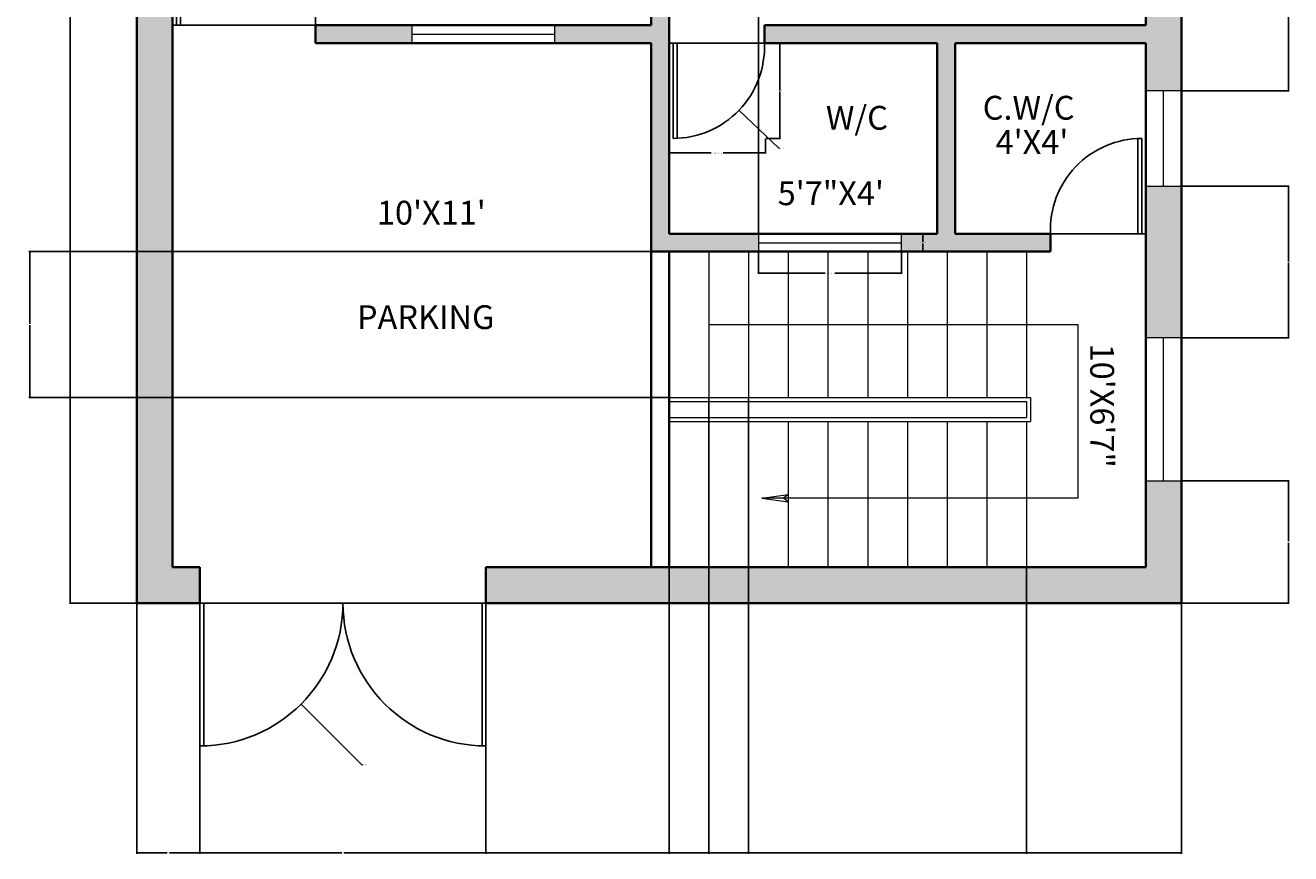
# Model space of a CAD drawing. Units: inches. Extents: x 2 to 321, y -521 to 41.
# Tile 1 of 2: x 2 to 321, y -521 to -312. Entities that reach past the tile are written whole.
import ezdxf

# ---------------------------------------------------------------- set-up
doc = ezdxf.new("R2010")
doc.units = ezdxf.units.IN
doc.header["$MEASUREMENT"] = 0
for name, color, linetype, lineweight in [('A-ANNO-DIMS', 2, 'Continuous', 18), ('A-ANNO-TEXT', 22, 'Continuous', 18), ('A-AREA-IDEN', 102, 'Continuous', 25), ('A-DOOR', 3, 'Continuous', 25), ('A-FLOR-STRS', 7, 'Continuous', 18), ('A-GLAZ', 4, 'Continuous', 18), ('A-WALL', 7, 'Continuous', 35), ('A-WALL-PATT', 5, 'Continuous', 13)]:
    doc.layers.add(name, color=color, linetype=linetype, lineweight=lineweight)
doc.styles.get("Standard").update_dxf_attribs({"font": 'arial.ttf'})
doc.dimstyles.get("Standard").update_dxf_attribs({"dimtxt": 0.18, "dimasz": 0.18, "dimexe": 0.18, "dimexo": 0.0625, "dimgap": 0.09, "dimtad": 0, "dimtih": 1, "dimtoh": 1, "dimdec": 0, "dimzin": 0, "dimdsep": 46, "dimlunit": 3, "dimtxsty": 'Standard', "dimcen": 0.09, "dimadec": 0, "dimazin": 0, "dimtfac": 1, "dimtdec": 0, "dimtofl": 0, "dimtmove": 0, "dimatfit": 3, "dimfxl": 1, "dimtolj": 1, "dimtzin": 0, "dimarcsym": 0})

# ---------------------------------------------------------------- blocks, each defined once
blk = doc.blocks.new('*D2')
at = {"layer": 'A-ANNO-DIMS', "color": 0, "lineweight": -2, "transparency": 16777216}
for p, q in [((30.1, 14.04), (13.23, 14.04)), ((13.41, 13.86), (13.41, -218.56)), ((13.41, -457.28), (13.41, -224.87)), ((30.1, -457.46), (13.23, -457.46))]:
    blk.add_line(p, q, dxfattribs=at)
at = {"layer": 'A-ANNO-DIMS', "color": 0, "transparency": 16777216}
for points in [[(13.38, 13.86), (13.44, 13.86), (13.41, 14.04)], [(13.38, -457.28), (13.44, -457.28), (13.41, -457.46)]]:
    blk.add_solid(points, dxfattribs=at)
at = {"layer": 'Defpoints', "color": 0, "transparency": 16777216}
for p in [(30.16, 14.04), (13.41, -457.46), (30.16, -457.46)]:
    blk.add_point(p, dxfattribs=at)
at = {"layer": 'A-ANNO-DIMS', "color": 0, "transparency": 16777216, "insert": (13.41, -221.71), "char_height": 6, "attachment_point": 5}
blk.add_mtext('\\A1;39\'-4"', dxfattribs=at)
blk = doc.blocks.new('WIN-36IN-9IN-WALL')
for p, q in [((0, 36), (0, 0)), ((9, 36), (0, 36)), ((4.5, 36), (4.5, 0)), ((9, 0), (9, 36)), ((0, 0), (9, 0))]:
    blk.add_line(p, q)
blk = doc.blocks.new('WIN-36IN-4_5IN-WALL')
for p, q in [((0, 4.5), (0, 0)), ((36, 4.5), (0, 4.5)), ((36, 0), (36, 4.5)), ((0, 2.25), (36, 2.25)), ((0, 0), (36, 0))]:
    blk.add_line(p, q)
blk = doc.blocks.new('WIN-24IN-9IN-WALL')
for p, q in [((0, 24), (0, 0)), ((9, 24), (0, 24)), ((4.5, 24), (4.5, 0)), ((9, 0), (9, 24)), ((0, 0), (9, 0))]:
    blk.add_line(p, q)
blk = doc.blocks.new('DOOR-SINGLE-36IN')
for p, q in [((1, 0), (1, 36)), ((2, 0), (2, 36)), ((36, 0), (0, 0))]:
    blk.add_line(p, q)
blk.add_arc((1, 0.99), 35.01, 358.3861, 90)
blk = doc.blocks.new('DOOR-SINGLE-24IN')
for p, q in [((24, 24), (0, 24)), ((1, 24), (1, 0)), ((2, 24), (2, 0))]:
    blk.add_line(p, q)
blk.add_arc((1, 23.02), 23.02, 270, 2.4378)
blk = doc.blocks.new('*D12')
at = {"layer": 'A-ANNO-DIMS', "color": 0, "lineweight": -2, "transparency": 16777216}
for p, q in [((186.66, -369.03), (186.66, -374.54)), ((222.66, -369.03), (222.66, -374.54)), ((186.84, -374.36), (203.43, -374.36)), ((222.48, -374.36), (205.88, -374.36))]:
    blk.add_line(p, q, dxfattribs=at)
at = {"layer": 'A-ANNO-DIMS', "color": 0, "transparency": 16777216}
for points in [[(186.84, -374.33), (186.84, -374.39), (186.66, -374.36)], [(222.48, -374.33), (222.48, -374.39), (222.66, -374.36)]]:
    blk.add_solid(points, dxfattribs=at)
at = {"layer": 'Defpoints', "color": 0, "transparency": 16777216}
for p in [(186.66, -368.96), (222.66, -368.96), (222.66, -374.36)]:
    blk.add_point(p, dxfattribs=at)
at = {"layer": 'A-ANNO-DIMS', "color": 0, "transparency": 16777216, "insert": (204.66, -374.36), "char_height": 0.18, "attachment_point": 5}
blk.add_mtext('\\A1;WINDOW 3\'-0" TYP.', dxfattribs=at)
blk = doc.blocks.new('*D13')
at = {"layer": 'A-ANNO-DIMS', "color": 0, "lineweight": -2, "transparency": 16777216}
for p, q in [((222.72, -364.46), (228.24, -364.46)), ((228.06, -364.64), (228.06, -366.53)), ((222.72, -368.96), (228.24, -368.96)), ((228.06, -368.78), (228.06, -366.9))]:
    blk.add_line(p, q, dxfattribs=at)
at = {"layer": 'A-ANNO-DIMS', "color": 0, "transparency": 16777216}
for points in [[(228.03, -364.64), (228.09, -364.64), (228.06, -364.46)], [(228.03, -368.78), (228.09, -368.78), (228.06, -368.96)]]:
    blk.add_solid(points, dxfattribs=at)
at = {"layer": 'Defpoints', "color": 0, "transparency": 16777216}
for p in [(222.66, -364.46), (228.06, -364.46), (222.66, -368.96)]:
    blk.add_point(p, dxfattribs=at)
at = {"layer": 'A-ANNO-DIMS', "color": 0, "transparency": 16777216, "insert": (228.06, -366.71), "char_height": 0.18, "attachment_point": 5}
blk.add_mtext('\\A1;0\'-4 1/2" TYP.', dxfattribs=at)
blk = doc.blocks.new('*D16')
at = {"layer": 'A-ANNO-DIMS', "color": 0, "lineweight": -2, "transparency": 16777216}
for p, q in [((164.16, -340.53), (164.16, -344.28)), ((188.43, -340.53), (188.43, -344.28)), ((164.34, -344.1), (174.79, -344.1)), ((188.25, -344.1), (177.8, -344.1))]:
    blk.add_line(p, q, dxfattribs=at)
at = {"layer": 'A-ANNO-DIMS', "color": 0, "transparency": 16777216}
for points in [[(164.34, -344.07), (164.34, -344.13), (164.16, -344.1)], [(188.25, -344.07), (188.25, -344.13), (188.43, -344.1)]]:
    blk.add_solid(points, dxfattribs=at)
at = {"layer": 'Defpoints', "color": 0, "transparency": 16777216}
for p in [(164.16, -340.46), (188.43, -340.46), (188.43, -344.1)]:
    blk.add_point(p, dxfattribs=at)
at = {"layer": 'A-ANNO-DIMS', "color": 0, "transparency": 16777216, "insert": (176.29, -344.1), "char_height": 0.18, "attachment_point": 5}
blk.add_mtext('\\A1;WC DOOR 2\'-0 1/2" TYP.', dxfattribs=at)
blk = doc.blocks.new('*D17')
at = {"layer": 'A-ANNO-DIMS', "color": 0, "lineweight": -2, "transparency": 16777216}
for p, q in [((188.49, -316.46), (192.25, -316.46)), ((192.07, -316.64), (192.07, -328.28)), ((192.07, -340.28), (192.07, -328.65)), ((188.49, -340.46), (192.25, -340.46))]:
    blk.add_line(p, q, dxfattribs=at)
at = {"layer": 'A-ANNO-DIMS', "color": 0, "transparency": 16777216}
for points in [[(192.04, -316.64), (192.1, -316.64), (192.07, -316.46)], [(192.04, -340.28), (192.1, -340.28), (192.07, -340.46)]]:
    blk.add_solid(points, dxfattribs=at)
at = {"layer": 'Defpoints', "color": 0, "transparency": 16777216}
for p in [(188.43, -316.46), (192.07, -316.46), (188.43, -340.46)]:
    blk.add_point(p, dxfattribs=at)
at = {"layer": 'A-ANNO-DIMS', "color": 0, "transparency": 16777216, "insert": (192.07, -328.46), "char_height": 0.18, "attachment_point": 5}
blk.add_mtext('\\A1;2\'-0" TYP.', dxfattribs=at)
blk = doc.blocks.new('*D18')
at = {"layer": 'A-ANNO-DIMS', "color": 0, "lineweight": -2, "transparency": 16777216}
for p, q in [((30.16, -457.53), (30.16, -520.59)), ((46.07, -457.53), (46.07, -520.59)), ((30.34, -520.41), (37.8, -520.41)), ((45.89, -520.41), (38.44, -520.41))]:
    blk.add_line(p, q, dxfattribs=at)
at = {"layer": 'A-ANNO-DIMS', "color": 0, "transparency": 16777216}
for points in [[(30.34, -520.38), (30.34, -520.44), (30.16, -520.41)], [(45.89, -520.38), (45.89, -520.44), (46.07, -520.41)]]:
    blk.add_solid(points, dxfattribs=at)
at = {"layer": 'Defpoints', "color": 0, "transparency": 16777216}
for p in [(30.16, -457.46), (46.07, -457.46), (46.07, -520.41)]:
    blk.add_point(p, dxfattribs=at)
at = {"layer": 'A-ANNO-DIMS', "color": 0, "transparency": 16777216, "insert": (38.12, -520.41), "char_height": 0.18, "attachment_point": 5}
blk.add_mtext('\\A1;1\'-4"', dxfattribs=at)
blk = doc.blocks.new('*D19')
at = {"layer": 'A-ANNO-DIMS', "color": 0, "lineweight": -2, "transparency": 16777216}
for p, q in [((46.07, -457.53), (46.07, -520.59)), ((118.07, -457.53), (118.07, -520.59)), ((46.25, -520.41), (81.75, -520.41)), ((117.89, -520.41), (82.4, -520.41))]:
    blk.add_line(p, q, dxfattribs=at)
at = {"layer": 'A-ANNO-DIMS', "color": 0, "transparency": 16777216}
for points in [[(46.25, -520.38), (46.25, -520.44), (46.07, -520.41)], [(117.89, -520.38), (117.89, -520.44), (118.07, -520.41)]]:
    blk.add_solid(points, dxfattribs=at)
at = {"layer": 'Defpoints', "color": 0, "transparency": 16777216}
for p in [(46.07, -457.46), (118.07, -457.46), (118.07, -520.41)]:
    blk.add_point(p, dxfattribs=at)
at = {"layer": 'A-ANNO-DIMS', "color": 0, "transparency": 16777216, "insert": (82.07, -520.41), "char_height": 0.18, "attachment_point": 5}
blk.add_mtext('\\A1;6\'-0"', dxfattribs=at)
blk = doc.blocks.new('*D20')
at = {"layer": 'A-ANNO-DIMS', "color": 0, "lineweight": -2, "transparency": 16777216}
for p, q in [((118.07, -457.53), (118.07, -520.59)), ((293.16, -457.53), (293.16, -520.59)), ((118.25, -520.41), (205.23, -520.41)), ((292.98, -520.41), (206.01, -520.41))]:
    blk.add_line(p, q, dxfattribs=at)
at = {"layer": 'A-ANNO-DIMS', "color": 0, "transparency": 16777216}
for points in [[(118.25, -520.38), (118.25, -520.44), (118.07, -520.41)], [(292.98, -520.38), (292.98, -520.44), (293.16, -520.41)]]:
    blk.add_solid(points, dxfattribs=at)
at = {"layer": 'Defpoints', "color": 0, "transparency": 16777216}
for p in [(118.07, -457.46), (293.16, -457.46), (293.16, -520.41)]:
    blk.add_point(p, dxfattribs=at)
at = {"layer": 'A-ANNO-DIMS', "color": 0, "transparency": 16777216, "insert": (205.62, -520.41), "char_height": 0.18, "attachment_point": 5}
blk.add_mtext('\\A1;14\'-7"', dxfattribs=at)
blk = doc.blocks.new('*D26')
at = {"layer": 'A-ANNO-DIMS', "color": 0, "lineweight": -2, "transparency": 16777216}
for p, q in [((293.22, -269.96), (320.29, -269.96)), ((320.11, -270.14), (320.11, -299.03)), ((320.11, -328.28), (320.11, -299.4)), ((293.22, -328.46), (320.29, -328.46))]:
    blk.add_line(p, q, dxfattribs=at)
at = {"layer": 'A-ANNO-DIMS', "color": 0, "transparency": 16777216}
for points in [[(320.08, -270.14), (320.14, -270.14), (320.11, -269.96)], [(320.08, -328.28), (320.14, -328.28), (320.11, -328.46)]]:
    blk.add_solid(points, dxfattribs=at)
at = {"layer": 'Defpoints', "color": 0, "transparency": 16777216}
for p in [(293.16, -269.96), (293.16, -328.46), (320.11, -328.46)]:
    blk.add_point(p, dxfattribs=at)
at = {"layer": 'A-ANNO-DIMS', "color": 0, "transparency": 16777216, "insert": (320.11, -299.21), "char_height": 0.18, "attachment_point": 5}
blk.add_mtext('\\A1;4\'-10 1/2"', dxfattribs=at)
blk = doc.blocks.new('*D27')
at = {"layer": 'A-ANNO-DIMS', "color": 0, "lineweight": -2, "transparency": 16777216}
for p, q in [((293.22, -352.46), (320.29, -352.46)), ((320.11, -352.64), (320.11, -371.41)), ((320.11, -390.53), (320.11, -371.77)), ((293.22, -390.71), (320.29, -390.71))]:
    blk.add_line(p, q, dxfattribs=at)
at = {"layer": 'A-ANNO-DIMS', "color": 0, "transparency": 16777216}
for points in [[(320.08, -352.64), (320.14, -352.64), (320.11, -352.46)], [(320.08, -390.53), (320.14, -390.53), (320.11, -390.71)]]:
    blk.add_solid(points, dxfattribs=at)
at = {"layer": 'Defpoints', "color": 0, "transparency": 16777216}
for p in [(293.16, -352.46), (293.16, -390.71), (320.11, -390.71)]:
    blk.add_point(p, dxfattribs=at)
at = {"layer": 'A-ANNO-DIMS', "color": 0, "transparency": 16777216, "insert": (320.11, -371.59), "char_height": 0.18, "attachment_point": 5}
blk.add_mtext('\\A1;3\'-2 1/2"', dxfattribs=at)
blk = doc.blocks.new('*D28')
at = {"layer": 'A-ANNO-DIMS', "color": 0, "lineweight": -2, "transparency": 16777216}
for p, q in [((293.22, -426.71), (320.29, -426.71)), ((320.11, -426.89), (320.11, -441.91)), ((320.11, -457.28), (320.11, -442.27)), ((293.22, -457.46), (320.29, -457.46))]:
    blk.add_line(p, q, dxfattribs=at)
at = {"layer": 'A-ANNO-DIMS', "color": 0, "transparency": 16777216}
for points in [[(320.08, -426.89), (320.14, -426.89), (320.11, -426.71)], [(320.08, -457.28), (320.14, -457.28), (320.11, -457.46)]]:
    blk.add_solid(points, dxfattribs=at)
at = {"layer": 'Defpoints', "color": 0, "transparency": 16777216}
for p in [(293.16, -426.71), (293.16, -457.46), (320.11, -457.46)]:
    blk.add_point(p, dxfattribs=at)
at = {"layer": 'A-ANNO-DIMS', "color": 0, "transparency": 16777216, "insert": (320.11, -442.09), "char_height": 0.18, "attachment_point": 5}
blk.add_mtext('\\A1;2\'-7"', dxfattribs=at)
blk = doc.blocks.new('*D30')
at = {"layer": 'A-ANNO-DIMS', "color": 0, "lineweight": -2, "transparency": 16777216}
for p, q in [((164.16, -364.4), (164.16, 41.17)), ((164.34, 40.99), (174.81, 40.99)), ((186.48, 40.99), (176.01, 40.99)), ((186.66, -364.4), (186.66, 41.17))]:
    blk.add_line(p, q, dxfattribs=at)
at = {"layer": 'A-ANNO-DIMS', "color": 0, "transparency": 16777216}
for points in [[(164.34, 41.02), (164.34, 40.96), (164.16, 40.99)], [(186.48, 41.02), (186.48, 40.96), (186.66, 40.99)]]:
    blk.add_solid(points, dxfattribs=at)
at = {"layer": 'Defpoints', "color": 0, "transparency": 16777216}
for p in [(186.66, 40.99), (164.16, -364.46), (186.66, -364.46)]:
    blk.add_point(p, dxfattribs=at)
at = {"layer": 'A-ANNO-DIMS', "color": 0, "transparency": 16777216, "insert": (175.41, 40.99), "char_height": 0.18, "attachment_point": 5}
blk.add_mtext('\\A1;1\'-10 1/2"', dxfattribs=at)
blk = doc.blocks.new('*D31')
at = {"layer": 'A-ANNO-DIMS', "color": 0, "lineweight": -2, "transparency": 16777216}
for p, q in [((164.16, -448.53), (164.16, -520.59)), ((254.16, -448.53), (254.16, -520.59)), ((164.34, -520.41), (208.83, -520.41)), ((253.98, -520.41), (209.49, -520.41))]:
    blk.add_line(p, q, dxfattribs=at)
at = {"layer": 'A-ANNO-DIMS', "color": 0, "transparency": 16777216}
for points in [[(164.34, -520.38), (164.34, -520.44), (164.16, -520.41)], [(253.98, -520.38), (253.98, -520.44), (254.16, -520.41)]]:
    blk.add_solid(points, dxfattribs=at)
at = {"layer": 'Defpoints', "color": 0, "transparency": 16777216}
for p in [(164.16, -448.46), (254.16, -448.46), (254.16, -520.41)]:
    blk.add_point(p, dxfattribs=at)
at = {"layer": 'A-ANNO-DIMS', "color": 0, "transparency": 16777216, "insert": (209.16, -520.41), "char_height": 0.18, "attachment_point": 5}
blk.add_mtext('\\A1;7\'-6"', dxfattribs=at)
blk = doc.blocks.new('*D32')
at = {"layer": 'A-ANNO-DIMS', "color": 0, "lineweight": -2, "transparency": 16777216}
for p, q in [((174.16, -405.78), (174.16, -520.59)), ((184.16, -405.78), (184.16, -520.59)), ((174.34, -520.41), (178.76, -520.41)), ((183.98, -520.41), (179.56, -520.41))]:
    blk.add_line(p, q, dxfattribs=at)
at = {"layer": 'A-ANNO-DIMS', "color": 0, "transparency": 16777216}
for points in [[(174.34, -520.38), (174.34, -520.44), (174.16, -520.41)], [(183.98, -520.38), (183.98, -520.44), (184.16, -520.41)]]:
    blk.add_solid(points, dxfattribs=at)
at = {"layer": 'Defpoints', "color": 0, "transparency": 16777216}
for p in [(174.16, -405.71), (184.16, -405.71), (184.16, -520.41)]:
    blk.add_point(p, dxfattribs=at)
at = {"layer": 'A-ANNO-DIMS', "color": 0, "transparency": 16777216, "insert": (179.16, -520.41), "char_height": 0.18, "attachment_point": 5}
blk.add_mtext('\\A1;0\'-10"', dxfattribs=at)
blk = doc.blocks.new('*D33')
at = {"layer": 'A-ANNO-DIMS', "color": 0, "lineweight": -2, "transparency": 16777216}
for p, q in [((164.1, -368.96), (3.03, -368.96)), ((3.21, -369.14), (3.21, -387.16)), ((3.21, -405.53), (3.21, -387.52)), ((164.1, -405.71), (3.03, -405.71))]:
    blk.add_line(p, q, dxfattribs=at)
at = {"layer": 'A-ANNO-DIMS', "color": 0, "transparency": 16777216}
for points in [[(3.18, -369.14), (3.24, -369.14), (3.21, -368.96)], [(3.18, -405.53), (3.24, -405.53), (3.21, -405.71)]]:
    blk.add_solid(points, dxfattribs=at)
at = {"layer": 'Defpoints', "color": 0, "transparency": 16777216}
for p in [(3.21, -368.96), (164.16, -368.96), (164.16, -405.71)]:
    blk.add_point(p, dxfattribs=at)
at = {"layer": 'A-ANNO-DIMS', "color": 0, "transparency": 16777216, "insert": (3.21, -387.34), "char_height": 0.18, "attachment_point": 5}
blk.add_mtext('\\A1;3\'-1"', dxfattribs=at)
blk = doc.blocks.new('*D37')
at = {"layer": 'A-ANNO-DIMS', "color": 0, "lineweight": -2, "transparency": 16777216}
for p, q in [((45.98, -457.46), (46.16, -457.46)), ((46.07, -457.55), (46.07, -457.37)), ((86.8, -498.19), (71.66, -483.05)), ((86.98, -498.19), (86.8, -498.19))]:
    blk.add_line(p, q, dxfattribs=at)
at = {"layer": 'A-ANNO-DIMS', "color": 0, "transparency": 16777216}
blk.add_solid([(71.68, -483.03), (71.64, -483.07), (71.53, -482.92)], dxfattribs=at)
at = {"layer": 'Defpoints', "color": 0, "transparency": 16777216}
for p in [(46.07, -457.46), (71.53, -482.92)]:
    blk.add_point(p, dxfattribs=at)
at = {"layer": 'A-ANNO-DIMS', "color": 0, "transparency": 16777216, "insert": (87.59, -498.19), "char_height": 0.18, "attachment_point": 5}
blk.add_mtext('\\A1;2X R3\'-0"', dxfattribs=at)
blk = doc.blocks.new('*D39')
at = {"layer": 'A-ANNO-DIMS', "color": 0, "lineweight": -2, "transparency": 16777216}
for p, q in [((165.07, -317.44), (165.25, -317.44)), ((165.16, -317.53), (165.16, -317.35)), ((191.75, -342.93), (181.91, -333.5)), ((191.93, -342.93), (191.75, -342.93))]:
    blk.add_line(p, q, dxfattribs=at)
at = {"layer": 'A-ANNO-DIMS', "color": 0, "transparency": 16777216}
blk.add_solid([(181.93, -333.47), (181.89, -333.52), (181.78, -333.37)], dxfattribs=at)
at = {"layer": 'Defpoints', "color": 0, "transparency": 16777216}
for p in [(165.16, -317.44), (181.78, -333.37)]:
    blk.add_point(p, dxfattribs=at)
at = {"layer": 'A-ANNO-DIMS', "color": 0, "transparency": 16777216, "insert": (192.61, -342.93), "char_height": 0.18, "attachment_point": 5}
blk.add_mtext('\\A1;3X R1\'-11"', dxfattribs=at)

msp = doc.modelspace()

# ---------------------------------------------------------------- hatches: boundary and pattern name
at = {"layer": 'A-WALL-PATT'}
h = msp.add_hatch(color=256, dxfattribs=at)
h.dxf.hatch_style = 1
h.paths.add_polyline_path([(39.16, 5.04), (123.16, 5.04), (123.16, -48.65), (127.66, -48.65), (127.66, 5.04), (159.66, 5.04), (159.66, -114.96), (127.66, -114.96), (127.66, -77.44), (123.16, -77.44), (123.16, -119.46), (164.16, -119.46), (164.16, 5.04), (284.16, 5.04), (284.16, -36.96), (293.16, -36.96), (293.16, 14.04), (30.16, 14.04), (30.16, -36.96), (39.16, -36.96)])
h.paths.add_polyline_path([(39.16, -205.49), (30.16, -205.49), (30.16, -457.46), (46.07, -457.46), (46.07, -448.46), (39.16, -448.46)])
h.paths.add_polyline_path([(39.16, -119.46), (87.16, -119.46), (87.16, -114.96), (39.16, -114.96), (39.16, -72.96), (30.16, -72.96), (30.16, -169.49), (39.16, -169.49)])
h.paths.add_polyline_path([(293.16, -165.46), (284.16, -165.46), (284.16, -187.46), (224.16, -187.46), (224.16, -114.96), (200.16, -114.96), (200.16, -119.46), (219.66, -119.46), (219.66, -187.46), (200.16, -187.46), (200.16, -191.96), (284.16, -191.96), (284.16, -233.96), (293.16, -233.96)])
h.paths.add_polyline_path([(293.16, -72.96), (284.16, -72.96), (284.16, -114.96), (248.16, -114.96), (248.16, -119.46), (284.16, -119.46), (284.16, -141.46), (293.16, -141.46)])
h.paths.add_polyline_path([(293.16, -269.96), (284.16, -269.96), (284.16, -311.96), (188.16, -311.96), (188.16, -316.46), (231.66, -316.46), (231.66, -364.46), (222.66, -364.46), (222.66, -368.96), (260.16, -368.96), (260.16, -364.46), (236.16, -364.46), (236.16, -316.46), (284.16, -316.46), (284.16, -328.46), (293.16, -328.46)])
h.paths.add_polyline_path([(186.66, -364.46), (164.16, -364.46), (164.16, -187.46), (159.66, -187.46), (159.66, -311.96), (135.41, -311.96), (135.41, -316.46), (159.66, -316.46), (159.66, -368.96), (186.66, -368.96)])
h.paths.add_polyline_path([(293.16, -426.71), (284.16, -426.71), (284.16, -448.46), (118.07, -448.46), (118.07, -457.46), (293.16, -457.46)])
h.paths.add_polyline_path([(99.41, -311.96), (75.16, -311.96), (75.16, -316.46), (99.41, -316.46)])
h.paths.add_polyline_path([(293.16, -352.46), (284.16, -352.46), (284.16, -364.46), (284.16, -368.96), (284.16, -390.71), (293.16, -390.71)])

# ---------------------------------------------------------------- linework, layer by layer
at = {"layer": 'A-DOOR'}
for p, q in [((118.07, -457.46), (46.07, -457.46)), ((46.07, -457.46), (46.07, -493.46)), ((47.07, -457.46), (47.07, -493.46)), ((117.07, -457.46), (117.07, -493.46)), ((118.07, -457.46), (118.07, -493.46))]:
    msp.add_line(p, q, dxfattribs=at)
for centre, start, end in [((46.07, -457.46), 270, 0), ((118.07, -457.46), 180, 270)]:
    msp.add_arc(centre, 36, start, end, dxfattribs=at)
at = {"layer": 'A-FLOR-STRS'}
for p, q in [((174.16, -368.96), (174.16, -405.71)), ((184.16, -368.96), (184.16, -405.71)), ((194.16, -368.96), (194.16, -405.71)), ((204.16, -368.96), (204.16, -405.71)), ((214.16, -368.96), (214.16, -405.71)), ((224.16, -368.96), (224.16, -405.71)), ((234.16, -368.96), (234.16, -405.71)), ((244.16, -368.96), (244.16, -405.71)), ((254.16, -368.96), (254.16, -405.71)), ((174.16, -387.34), (267.05, -387.34)), ((267.05, -387.34), (267.05, -431.03)), ((164.16, -405.71), (255.16, -405.71)), ((164.16, -406.71), (254.16, -406.71)), ((254.16, -406.71), (254.16, -410.71)), ((255.16, -405.71), (255.16, -411.71)), ((164.16, -410.71), (254.16, -410.71)), ((164.16, -411.71), (255.16, -411.71)), ((174.16, -411.71), (174.16, -448.46)), ((184.16, -411.71), (184.16, -448.46)), ((194.16, -411.71), (194.16, -448.46)), ((204.16, -411.71), (204.16, -448.46)), ((214.16, -411.71), (214.16, -448.46)), ((224.16, -411.71), (224.16, -448.46)), ((234.16, -411.71), (234.16, -448.46)), ((244.16, -411.71), (244.16, -448.46)), ((254.16, -411.71), (254.16, -448.46)), ((187.55, -431.03), (194.16, -430.09)), ((267.05, -431.03), (187.55, -431.03)), ((187.55, -431.03), (194.16, -431.96)), ((194.16, -430.09), (192.94, -431.03)), ((194.16, -431.96), (192.94, -431.03))]:
    msp.add_line(p, q, dxfattribs=at)
at = {"layer": 'A-WALL'}
for p, q in [((30.16, 14.04), (30.16, -457.46)), ((293.16, 14.04), (293.16, -457.46)), ((39.16, -119.46), (39.16, -448.46)), ((159.66, -187.46), (159.66, -311.96)), ((164.16, -187.46), (164.16, -364.46)), ((284.16, -191.96), (284.16, -311.96)), ((75.16, -311.96), (159.66, -311.96)), ((75.16, -311.96), (75.16, -316.46)), ((188.16, -311.96), (284.16, -311.96)), ((188.16, -311.96), (188.16, -316.46)), ((75.16, -316.46), (159.66, -316.46)), ((159.66, -316.46), (159.66, -448.46)), ((188.16, -316.46), (231.66, -316.46)), ((231.66, -316.46), (231.66, -364.46)), ((236.16, -316.46), (236.16, -364.46)), ((236.16, -316.46), (284.16, -316.46)), ((284.16, -316.46), (284.16, -364.46)), ((164.16, -364.46), (231.66, -364.46)), ((236.16, -364.46), (260.16, -364.46)), ((260.16, -364.46), (260.16, -368.96)), ((284.16, -364.46), (284.16, -368.96)), ((159.66, -368.96), (260.16, -368.96)), ((164.16, -368.96), (164.16, -448.46)), ((284.16, -368.96), (284.16, -448.46)), ((39.16, -448.46), (46.07, -448.46)), ((46.07, -448.46), (46.07, -457.46)), ((118.07, -457.46), (118.07, -448.46)), ((118.07, -448.46), (284.16, -448.46)), ((30.16, -457.46), (46.07, -457.46)), ((118.07, -457.46), (293.16, -457.46))]:
    msp.add_line(p, q, dxfattribs=at)

# ---------------------------------------------------------------- block references
at = {"layer": 'A-DOOR'}
for name, p in [('DOOR-SINGLE-36IN', (39.16, -311.96)), ('DOOR-SINGLE-24IN', (164.16, -340.46))]:
    msp.add_blockref(name, p, dxfattribs=at)
at = {"layer": 'A-DOOR', "rotation": 180}
msp.add_blockref('DOOR-SINGLE-24IN', (284.16, -340.46), dxfattribs=at)
at = {"layer": 'A-GLAZ'}
for p in [(99.41, -316.46), (186.66, -368.96)]:
    msp.add_blockref('WIN-36IN-4_5IN-WALL', p, dxfattribs=at)
at = {"layer": 'A-GLAZ', "rotation": 180}
for name, p in [('WIN-24IN-9IN-WALL', (293.16, -328.46)), ('WIN-36IN-9IN-WALL', (293.16, -390.71))]:
    msp.add_blockref(name, p, dxfattribs=at)

# ---------------------------------------------------------------- texts
at = {"layer": 'A-ANNO-TEXT', "char_height": 6, "attachment_point": 1}
for s, insert in [("4'X4'", (246.34, -338.35)), ('5\'7"X4\'', (191.5, -351.26)), ("10'X11'", (90.62, -356.16))]:
    msp.add_mtext(s, dxfattribs=dict(at, insert=insert))
at = {"layer": 'A-ANNO-TEXT', "insert": (276.18, -392.13), "char_height": 6, "attachment_point": 1, "rotation": 270}
msp.add_mtext_dynamic_manual_height_columns('10\'X6\'7"', width=0.3931, gutter_width=1, heights=[0], dxfattribs=at)
at = {"layer": 'A-AREA-IDEN', "char_height": 6, "attachment_point": 1}
for s, insert in [('C.W/C', (243.11, -329.73)), ('W/C', (203.63, -332.26)), ('PARKING', (85.59, -382.47))]:
    msp.add_mtext(s, dxfattribs=dict(at, insert=insert))

# ---------------------------------------------------------------- dimensions: what is measured, and where the dimension line sits
at = {"layer": 'A-ANNO-DIMS'}
for base, p1, p2, picture, middle in [((186.66, 40.99), (164.16, -364.46), (186.66, -364.46), '*D30', (175.41, 40.99)), ((184.16, -520.41), (174.16, -405.71), (184.16, -405.71), '*D32', (179.16, -520.41)), ((254.16, -520.41), (164.16, -448.46), (254.16, -448.46), '*D31', (209.16, -520.41)), ((46.07, -520.41), (30.16, -457.46), (46.07, -457.46), '*D18', (38.12, -520.41)), ((118.07, -520.41), (46.07, -457.46), (118.07, -457.46), '*D19', (82.07, -520.41)), ((293.16, -520.41), (118.07, -457.46), (293.16, -457.46), '*D20', (205.62, -520.41))]:
    dim = msp.add_linear_dim(base=base, p1=p1, p2=p2, dimstyle='Standard', override={"dimdec": 1, "dimlfac": 1, "dimrnd": 0, "dimzin": 1, "dimdsep": 46, "dimlunit": 4, "dimfrac": 2}, dxfattribs=at)
    dim.commit()
    dim.dimension.update_dxf_attribs({"geometry": picture, "text_midpoint": middle})
for base, p1, p2, override, picture, middle in [((13.41474495, -457.46394712), (30.16063488, 14.03605288), (30.16063488, -457.46394712), {"dimtxt": 6, "dimclrd": 0, "dimclre": 0, "dimclrt": 0}, '*D2', (13.41474495, -221.71394712)), ((320.11, -328.46), (293.16, -269.96), (293.16, -328.46), {"dimdec": 1, "dimlfac": 1, "dimrnd": 0, "dimzin": 1, "dimdsep": 46, "dimlunit": 4, "dimfrac": 2}, '*D26', (320.11, -299.21)), ((320.110635, -390.713947), (293.160635, -352.463947), (293.160635, -390.713947), {"dimdec": 1, "dimlfac": 1, "dimrnd": 0, "dimzin": 1, "dimdsep": 46, "dimlunit": 4, "dimfrac": 2}, '*D27', (320.110635, -371.588947)), ((3.210635, -368.963947), (164.160635, -405.713947), (164.160635, -368.963947), {"dimdec": 1, "dimlfac": 1, "dimrnd": 0, "dimzin": 1, "dimdsep": 46, "dimlunit": 4, "dimfrac": 2}, '*D33', (3.210635, -387.338947)), ((320.110635, -457.463947), (293.160635, -426.713947), (293.160635, -457.463947), {"dimdec": 1, "dimlfac": 1, "dimrnd": 0, "dimzin": 1, "dimdsep": 46, "dimlunit": 4, "dimfrac": 2}, '*D28', (320.110635, -442.088947))]:
    dim = msp.add_linear_dim(base=base, p1=p1, p2=p2, angle=90, dimstyle='Standard', override=override, dxfattribs=at)
    dim.commit()
    dim.dimension.update_dxf_attribs({"geometry": picture, "text_midpoint": middle})
for center, mpoint, text, picture, middle in [((165.16, -317.44), (181.78, -333.37), '3X <>', '*D39', (192.61, -342.93)), ((46.07, -457.46), (71.53, -482.92), '2X <>', '*D37', (87.59, -498.19))]:
    dim = msp.add_radius_dim(center=center, mpoint=mpoint, text=text, dimstyle='Standard', override={"dimdec": 1, "dimlfac": 1, "dimrnd": 0, "dimzin": 1, "dimdsep": 46, "dimlunit": 4, "dimfrac": 2}, dxfattribs=at)
    dim.commit()
    dim.dimension.update_dxf_attribs({"geometry": picture, "text_midpoint": middle, "dimtype": 164})
for base, p1, p2, picture, middle in [((192.07, -316.46), (188.43, -340.46), (188.43, -316.46), '*D17', (192.07, -328.46)), ((228.06, -364.46), (222.66, -368.96), (222.66, -364.46), '*D13', (228.06, -366.71))]:
    dim = msp.add_linear_dim(base=base, p1=p1, p2=p2, angle=90, text='<> TYP.', dimstyle='Standard', override={"dimdec": 1, "dimlfac": 1, "dimrnd": 0, "dimzin": 1, "dimdsep": 46, "dimlunit": 4, "dimfrac": 2}, dxfattribs=at)
    dim.commit()
    dim.dimension.update_dxf_attribs({"geometry": picture, "text_midpoint": middle})
for base, p1, p2, text, picture, middle in [((188.43, -344.1), (164.16, -340.46), (188.43, -340.46), 'WC DOOR <> TYP.', '*D16', (176.29, -344.1)), ((222.66, -374.36), (186.66, -368.96), (222.66, -368.96), 'WINDOW <> TYP.', '*D12', (204.66, -374.36))]:
    dim = msp.add_linear_dim(base=base, p1=p1, p2=p2, text=text, dimstyle='Standard', override={"dimdec": 1, "dimlfac": 1, "dimrnd": 0, "dimzin": 1, "dimdsep": 46, "dimlunit": 4, "dimfrac": 2}, dxfattribs=at)
    dim.commit()
    dim.dimension.update_dxf_attribs({"geometry": picture, "text_midpoint": middle})

doc.saveas('drawing.dxf')
